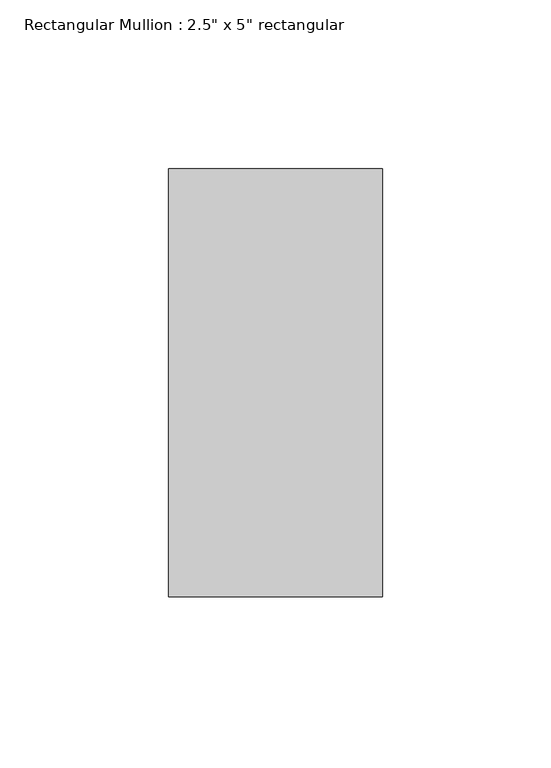
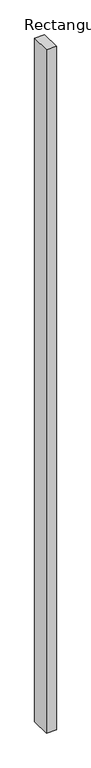
"""IFC4 building model written with IfcOpenShell, lengths in millimetres: member geometry."""

from ifc_helpers import new_model, si_unit, frame, origin, place, context, project, spatial, polyline, outline, extrude, source, transform, mapped, element, save


def member_50e41c3e(model_context):
    return source(origin(), model_context, "Body", "SweptSolid", [
        extrude(outline(polyline([(0.0, 63.5), (0.0, -63.5), (-63.5, -63.5), (-63.5, 63.5), (0.0, 63.5)])), frame((0.0, 0.0, -4564.4367512), z_axis=(0.0, 0.0, 1.0), x_axis=(1.0, 0.0, 0.0)), (0.0, 0.0, 1.0), 4564.4367512),
    ])


if __name__ == "__main__":
    model = new_model("IFC4")
    model_context = context("Model", 3, world=origin())
    ifc_project = project(units=[si_unit("LENGTHUNIT", "METRE", prefix="MILLI")], contexts=[model_context])
    site = spatial("IfcSite", under=ifc_project)
    building = spatial("IfcBuilding", under=site)
    placement = place(None, origin())
    member_shape = member_50e41c3e(model_context)
    element("IfcMember", 1, ObjectType="Rectangular Mullion : 2.5\" x 5\" rectangular", at=placement, inside=building, context=model_context, shape_type="MappedRepresentation", body=[
        mapped(member_shape, transform((0.0, 0.0, 0.0), x_axis=(1.0, 0.0, 0.0), y_axis=(0.0, 1.0, 0.0), z_axis=(0.0, 0.0, 1.0))),
    ])
    save(model, "model.ifc")

# Revit data of these elements
# Type "Rectangular Mullion : 2.5\" x 5\" rectangular"
#   built-in parameter 1007304 = 0.416667 (stored number, unit not read)
#   built-in parameter 1007301 = 0.104167 (stored number, unit not read)
#   built-in parameter 1007300 = 0.104167 (stored number, unit not read)
# Element 1 (IfcMember, "Rectangular Mullion : 2.5\" x 5\" rectangular")
#   Materials on its faces: "Aluminum"
# Materials
#   "Aluminum": class "Metal", colour RGB 247 247 247, transparency 0, Description = "Aluminum 6061", Cost = 0
